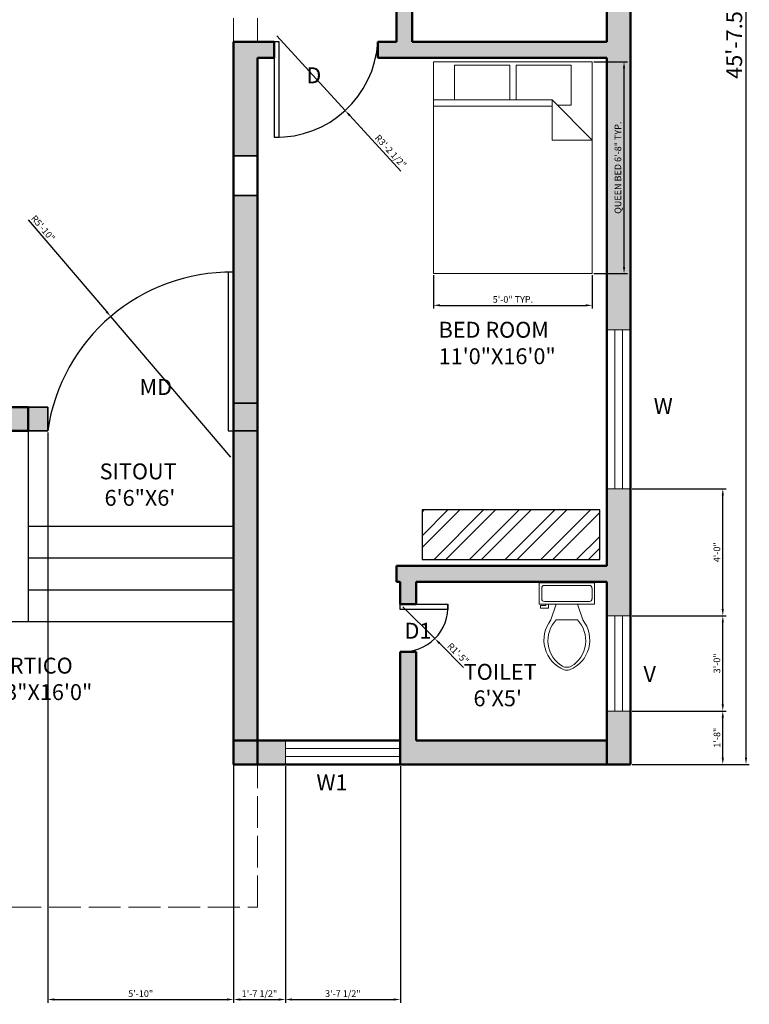
# Model space of a CAD drawing. Units: inches. Extents: x 5703 to 6226, y 10088 to 10813.
# Tile 2 of 5: x 5950 to 6226, y 10088 to 10460. Entities that reach past the tile are written whole.
import ezdxf

# ---------------------------------------------------------------- set-up
doc = ezdxf.new("R2010")
doc.units = ezdxf.units.IN
doc.linetypes.add('ACAD_ISO02W100', pattern=[15, 12, -3])
for name, color, linetype, lineweight in [('A-ANNO-DIMS', 2, 'Continuous', 18), ('A-ANNO-TEXT', 7, 'Continuous', 18), ('A-AREA-IDEN', 7, 'Continuous', 18), ('A-COLS', 7, 'Continuous', 35), ('A-COLS-PATT', 7, 'Continuous', 13), ('A-DOOR', 140, 'Continuous', 25), ('A-FLOR-CASE', 8, 'Continuous', 25), ('A-FLOR-CASE-PATT', 9, 'Continuous', 13), ('A-FLOR-FIXT', 8, 'Continuous', 18), ('A-FLOR-STRS', 7, 'Continuous', 25), ('A-FURN', 8, 'Continuous', 18), ('A-WALL', 7, 'Continuous', 50), ('A-WALL-PATT', 9, 'Continuous', 13)]:
    doc.layers.add(name, color=color, linetype=linetype, lineweight=lineweight)
for name, color, linetype, lineweight, true_color in [('A-GLAZ', 112, 'Continuous', 18, 0x1ce368), ('A-ROOF-OVHD', 30, 'ACAD_ISO02W100', 18, 0xf8991e), ('A-WALL-OVHD', 30, 'ACAD_ISO02W100', 18, 0xf8991e)]:
    doc.layers.add(name, color=color, linetype=linetype, lineweight=lineweight, true_color=true_color)
doc.styles.get("Standard").update_dxf_attribs({"font": 'arial.ttf'})
doc.dimstyles.new('ISO-25', dxfattribs={"dimtxt": 2.5, "dimasz": 2.5, "dimexe": 1.25, "dimexo": 0.625, "dimtad": 1, "dimlunit": 3, "dimtxsty": 'Standard', "dimcen": 2.5, "dimadec": 0, "dimazin": 0, "dimtfac": 1, "dimtmove": 0, "dimatfit": 3, "dimfxl": 1, "dimarcsym": 0})

# ---------------------------------------------------------------- blocks, each defined once
blk = doc.blocks.new('*D11')
at = {"layer": 'A-ANNO-DIMS', "color": 0, "lineweight": -2, "transparency": 16777216}
for p, q in [((6181.8, 10725.87), (6226.04, 10725.87)), ((6224.79, 10723.37), (6224.79, 10180.87)), ((6181.8, 10178.37), (6226.04, 10178.37))]:
    blk.add_line(p, q, dxfattribs=at)
at = {"layer": 'A-ANNO-DIMS', "color": 0, "transparency": 16777216}
for points in [[(6224.38, 10723.37), (6225.21, 10723.37), (6224.79, 10725.87)], [(6224.38, 10180.87), (6225.21, 10180.87), (6224.79, 10178.37)]]:
    blk.add_solid(points, dxfattribs=at)
at = {"layer": 'Defpoints', "color": 0, "transparency": 16777216}
for p in [(6181.18, 10725.87), (6181.18, 10178.37), (6224.79, 10178.37)]:
    blk.add_point(p, dxfattribs=at)
at = {"layer": 'A-ANNO-DIMS', "color": 0, "transparency": 16777216, "insert": (6221.12, 10452.12), "char_height": 6, "width": 12.5074, "attachment_point": 5, "rotation": 90}
blk.add_mtext('45\'-7.5"', dxfattribs=at)
blk = doc.blocks.new('Bed - Queen')
for p, q in [((0, -80.00003), (0, 0)), ((0, 0), (59.99999, 0)), ((59.99999, 0), (59.99999, -80.00003)), ((7.99999, -1.2), (28.79998, -1.2)), ((7.99999, -14.4), (7.99999, -1.2)), ((28.79998, -1.2), (28.79998, -14.4)), ((31.19999, -1.2), (51.99999, -1.2)), ((31.19999, -14.4), (31.19999, -1.2)), ((51.99999, -1.2), (51.99999, -16.4)), ((0, -14.4), (44.8, -14.4)), ((59.99999, -29.6), (44.8, -14.4)), ((44.8, -14.4), (44.8, -29.6)), ((44.8, -16.8), (0, -16.8)), ((51.99999, -16.4), (46.79936, -16.4)), ((44.8, -29.6), (59.99999, -29.6)), ((59.99999, -80.00003), (0, -80.00003))]:
    blk.add_line(p, q)
blk = doc.blocks.new('Toilet - top')
for p, q in [((9.5, -6), (9.5, -2)), ((-10, -8.5), (-8, -8.5)), ((-10, -9.5), (-10, -8.5)), ((-7, -9.5), (-10, -9.5)), ((-8, -8.5), (-8, -8)), ((-7, -8), (-7, -9.5)), ((-4, -8), (-6, -14)), ((4, -8), (6, -14)), ((4, -14), (-4, -14))]:
    blk.add_line(p, q)
blk.add_lwpolyline([(10.5, -8), (10.5, 0), (-10.5, 0), (-10.5, -8)], close=True)
for points in [[(-9.5, -2), (-9.5, -6)], [(8.5, -1), (-8.5, -1)], [(-8.5, -7), (8.5, -7)]]:
    blk.add_lwpolyline(points)
for centre, radius, start, end in [((-8.62, -1.88), 0.884, 81.8699, 188.1301), ((8.62, -1.88), 0.884, 351.8699, 98.1301), ((-8.62, -6.12), 0.884, 171.8699, 278.1301), ((8.62, -6.12), 0.884, 261.8699, 8.1301), ((3.52, -21.58), 12.17, 141.4691, 247.9714), ((4.2, -21.82), 11.33, 136.3677, 238.9468), ((-3.52, -21.58), 12.17, 292.0284, 38.5307), ((-4.2, -21.82), 11.33, 301.053, 43.6321), ((0, -27.88), 4, 245.7318, 294.2682), ((0, -29), 4, 254.8605, 285.1395)]:
    blk.add_arc(centre, radius, start, end)
blk = doc.blocks.new('WIN-60x9')
for p, q in [((9, 60), (0, 60)), ((0, 60), (0, 0)), ((3, 60), (3, 0)), ((6, 0), (6, 60)), ((9, 0), (9, 60)), ((0, 0), (9, 0))]:
    blk.add_line(p, q)
blk = doc.blocks.new('*D18')
at = {"layer": 'A-ANNO-DIMS', "color": 0, "lineweight": -2, "transparency": 16777216}
for p, q in [((6167.33, 10443.83), (6179.96, 10443.83)), ((6178.71, 10366.33), (6178.71, 10441.33)), ((6167.33, 10363.83), (6179.96, 10363.83))]:
    blk.add_line(p, q, dxfattribs=at)
at = {"layer": 'A-ANNO-DIMS', "color": 0, "transparency": 16777216}
for points in [[(6178.29, 10441.33), (6179.13, 10441.33), (6178.71, 10443.83)], [(6178.29, 10366.33), (6179.13, 10366.33), (6178.71, 10363.83)]]:
    blk.add_solid(points, dxfattribs=at)
at = {"layer": 'Defpoints', "color": 0, "transparency": 16777216}
for p in [(6166.71, 10443.83), (6178.71, 10443.83), (6166.71, 10363.83)]:
    blk.add_point(p, dxfattribs=at)
at = {"layer": 'A-ANNO-DIMS', "color": 0, "transparency": 16777216, "insert": (6176.71, 10403.83), "char_height": 2.5, "attachment_point": 5, "rotation": 90}
blk.add_mtext('QUEEN BED 6\'-8" TYP.', dxfattribs=at)
blk = doc.blocks.new('*D19')
at = {"layer": 'A-ANNO-DIMS', "color": 0, "lineweight": -2, "transparency": 16777216}
for p, q in [((6106.71, 10363.21), (6106.71, 10350.58)), ((6166.71, 10363.21), (6166.71, 10350.58)), ((6109.21, 10351.83), (6164.21, 10351.83))]:
    blk.add_line(p, q, dxfattribs=at)
at = {"layer": 'A-ANNO-DIMS', "color": 0, "transparency": 16777216}
for points in [[(6109.21, 10352.25), (6109.21, 10351.42), (6106.71, 10351.83)], [(6164.21, 10352.25), (6164.21, 10351.42), (6166.71, 10351.83)]]:
    blk.add_solid(points, dxfattribs=at)
at = {"layer": 'Defpoints', "color": 0, "transparency": 16777216}
for p in [(6106.71, 10363.83), (6166.71, 10363.83), (6166.71, 10351.83)]:
    blk.add_point(p, dxfattribs=at)
at = {"layer": 'A-ANNO-DIMS', "color": 0, "transparency": 16777216, "insert": (6136.71, 10353.73), "char_height": 2.5, "attachment_point": 5}
blk.add_mtext('5\'-0" TYP.', dxfattribs=at)
blk = doc.blocks.new('*D42')
at = {"layer": 'A-ANNO-DIMS', "color": 0, "lineweight": -2, "transparency": 16777216}
for p, q in [((5960.95, 10303.74), (5960.95, 10088.29)), ((6031.18, 10303.74), (6031.18, 10088.29)), ((5963.45, 10089.54), (6028.68, 10089.54))]:
    blk.add_line(p, q, dxfattribs=at)
at = {"layer": 'A-ANNO-DIMS', "color": 0, "transparency": 16777216}
for points in [[(5963.45, 10089.96), (5963.45, 10089.12), (5960.95, 10089.54)], [(6028.68, 10089.96), (6028.68, 10089.12), (6031.18, 10089.54)]]:
    blk.add_solid(points, dxfattribs=at)
at = {"layer": 'Defpoints', "color": 0, "transparency": 16777216}
for p in [(5960.95, 10304.37), (6031.18, 10304.37), (6031.18, 10089.54)]:
    blk.add_point(p, dxfattribs=at)
at = {"layer": 'A-ANNO-DIMS', "color": 0, "transparency": 16777216, "insert": (5996.07, 10091.44), "char_height": 2.5, "attachment_point": 5}
blk.add_mtext('5\'-10"', dxfattribs=at)
blk = doc.blocks.new('*D51')
at = {"layer": 'A-ANNO-DIMS', "color": 0, "lineweight": -2, "transparency": 16777216}
for p, q in [((6181.8, 10198.55), (6217.28, 10198.55)), ((6216.03, 10180.87), (6216.03, 10196.05)), ((6181.8, 10178.37), (6217.28, 10178.37))]:
    blk.add_line(p, q, dxfattribs=at)
at = {"layer": 'A-ANNO-DIMS', "color": 0, "transparency": 16777216}
for points in [[(6215.61, 10196.05), (6216.44, 10196.05), (6216.03, 10198.55)], [(6215.61, 10180.87), (6216.44, 10180.87), (6216.03, 10178.37)]]:
    blk.add_solid(points, dxfattribs=at)
at = {"layer": 'Defpoints', "color": 0, "transparency": 16777216}
for p in [(6181.18, 10198.55), (6216.03, 10198.55), (6181.18, 10178.37)]:
    blk.add_point(p, dxfattribs=at)
at = {"layer": 'A-ANNO-DIMS', "color": 0, "transparency": 16777216, "insert": (6214.12, 10188.46), "char_height": 2.5, "attachment_point": 5, "rotation": 90}
blk.add_mtext('1\'-8"', dxfattribs=at)
blk = doc.blocks.new('*D52')
at = {"layer": 'A-ANNO-DIMS', "color": 0, "lineweight": -2, "transparency": 16777216}
for p, q in [((6181.8, 10234.55), (6217.28, 10234.55)), ((6216.03, 10201.05), (6216.03, 10232.05)), ((6181.8, 10198.55), (6217.28, 10198.55))]:
    blk.add_line(p, q, dxfattribs=at)
at = {"layer": 'A-ANNO-DIMS', "color": 0, "transparency": 16777216}
for points in [[(6215.61, 10232.05), (6216.44, 10232.05), (6216.03, 10234.55)], [(6215.61, 10201.05), (6216.44, 10201.05), (6216.03, 10198.55)]]:
    blk.add_solid(points, dxfattribs=at)
at = {"layer": 'Defpoints', "color": 0, "transparency": 16777216}
for p in [(6181.18, 10234.55), (6216.03, 10234.55), (6181.18, 10198.55)]:
    blk.add_point(p, dxfattribs=at)
at = {"layer": 'A-ANNO-DIMS', "color": 0, "transparency": 16777216, "insert": (6214.12, 10216.55), "char_height": 2.5, "attachment_point": 5, "rotation": 90}
blk.add_mtext('3\'-0"', dxfattribs=at)
blk = doc.blocks.new('*D53')
at = {"layer": 'A-ANNO-DIMS', "color": 0, "lineweight": -2, "transparency": 16777216}
for p, q in [((6181.8, 10282.53), (6217.28, 10282.53)), ((6216.03, 10237.05), (6216.03, 10280.03)), ((6181.8, 10234.55), (6217.28, 10234.55))]:
    blk.add_line(p, q, dxfattribs=at)
at = {"layer": 'A-ANNO-DIMS', "color": 0, "transparency": 16777216}
for points in [[(6215.61, 10280.03), (6216.44, 10280.03), (6216.03, 10282.53)], [(6215.61, 10237.05), (6216.44, 10237.05), (6216.03, 10234.55)]]:
    blk.add_solid(points, dxfattribs=at)
at = {"layer": 'Defpoints', "color": 0, "transparency": 16777216}
for p in [(6181.18, 10282.53), (6216.03, 10282.53), (6181.18, 10234.55)]:
    blk.add_point(p, dxfattribs=at)
at = {"layer": 'A-ANNO-DIMS', "color": 0, "transparency": 16777216, "insert": (6214.12, 10258.54), "char_height": 2.5, "attachment_point": 5, "rotation": 90}
blk.add_mtext('4\'-0"', dxfattribs=at)
blk = doc.blocks.new('*D55')
at = {"layer": 'A-ANNO-DIMS', "color": 0, "lineweight": -2, "transparency": 16777216}
for p, q in [((6031.18, 10177.74), (6031.18, 10088.29)), ((6050.75, 10177.74), (6050.75, 10088.29)), ((6033.68, 10089.54), (6048.25, 10089.54))]:
    blk.add_line(p, q, dxfattribs=at)
at = {"layer": 'A-ANNO-DIMS', "color": 0, "transparency": 16777216}
for points in [[(6033.68, 10089.96), (6033.68, 10089.12), (6031.18, 10089.54)], [(6048.25, 10089.96), (6048.25, 10089.12), (6050.75, 10089.54)]]:
    blk.add_solid(points, dxfattribs=at)
at = {"layer": 'Defpoints', "color": 0, "transparency": 16777216}
for p in [(6031.18, 10178.37), (6050.75, 10178.37), (6050.75, 10089.54)]:
    blk.add_point(p, dxfattribs=at)
at = {"layer": 'A-ANNO-DIMS', "color": 0, "transparency": 16777216, "insert": (6040.96, 10091.46), "char_height": 2.5, "attachment_point": 5}
blk.add_mtext('1\'-7 1/2"', dxfattribs=at)
blk = doc.blocks.new('*D56')
at = {"layer": 'A-ANNO-DIMS', "color": 0, "lineweight": -2, "transparency": 16777216}
for p, q in [((6050.75, 10177.74), (6050.75, 10088.29)), ((6094.18, 10177.74), (6094.18, 10088.29)), ((6053.25, 10089.54), (6091.68, 10089.54))]:
    blk.add_line(p, q, dxfattribs=at)
at = {"layer": 'A-ANNO-DIMS', "color": 0, "transparency": 16777216}
for points in [[(6053.25, 10089.96), (6053.25, 10089.12), (6050.75, 10089.54)], [(6091.68, 10089.96), (6091.68, 10089.12), (6094.18, 10089.54)]]:
    blk.add_solid(points, dxfattribs=at)
at = {"layer": 'Defpoints', "color": 0, "transparency": 16777216}
for p in [(6050.75, 10178.37), (6094.18, 10178.37), (6094.18, 10089.54)]:
    blk.add_point(p, dxfattribs=at)
at = {"layer": 'A-ANNO-DIMS', "color": 0, "transparency": 16777216, "insert": (6072.46, 10091.46), "char_height": 2.5, "attachment_point": 5}
blk.add_mtext('3\'-7 1/2"', dxfattribs=at)
blk = doc.blocks.new('*D60')
at = {"layer": 'A-ANNO-DIMS', "color": 0, "lineweight": -2, "transparency": 16777216}
for p, q in [((6047.46, 10453.63), (6073.34, 10425.44)), ((6094.33, 10402.58), (6075.04, 10423.6))]:
    blk.add_line(p, q, dxfattribs=at)
at = {"layer": 'A-ANNO-DIMS', "color": 0, "transparency": 16777216}
blk.add_solid([(6075.34, 10423.88), (6074.73, 10423.31), (6073.34, 10425.44)], dxfattribs=at)
at = {"layer": 'Defpoints', "color": 0, "transparency": 16777216}
for p in [(6047.46, 10453.63), (6073.34, 10425.44)]:
    blk.add_point(p, dxfattribs=at)
at = {"layer": 'A-ANNO-DIMS', "color": 0, "transparency": 16777216, "insert": (6090.29, 10409.82), "char_height": 2.5, "attachment_point": 5, "rotation": 312.5558}
blk.add_mtext('R3\'-2 1/2"', dxfattribs=at)
blk = doc.blocks.new('*D61')
at = {"layer": 'A-ANNO-DIMS', "color": 0, "lineweight": -2, "transparency": 16777216}
for p, q in [((6095.18, 10237.95), (6107.22, 10225.91)), ((6118.08, 10215.05), (6108.99, 10224.15))]:
    blk.add_line(p, q, dxfattribs=at)
at = {"layer": 'A-ANNO-DIMS', "color": 0, "transparency": 16777216}
blk.add_solid([(6109.28, 10224.44), (6108.69, 10223.85), (6107.22, 10225.91)], dxfattribs=at)
at = {"layer": 'Defpoints', "color": 0, "transparency": 16777216}
for p in [(6095.18, 10237.95), (6107.22, 10225.91)]:
    blk.add_point(p, dxfattribs=at)
at = {"layer": 'A-ANNO-DIMS', "color": 0, "transparency": 16777216, "insert": (6115.79, 10220.03), "char_height": 2.5, "attachment_point": 5, "rotation": 315.0011}
blk.add_mtext('R1\'-5"', dxfattribs=at)
blk = doc.blocks.new('*D62')
at = {"layer": 'A-ANNO-DIMS', "color": 0, "lineweight": -2, "transparency": 16777216}
for p, q in [((5953.52, 10384.16), (5983.13, 10349.51)), ((6030.18, 10294.45), (5984.75, 10347.61))]:
    blk.add_line(p, q, dxfattribs=at)
at = {"layer": 'A-ANNO-DIMS', "color": 0, "transparency": 16777216}
blk.add_solid([(5983.44, 10349.78), (5982.81, 10349.24), (5984.75, 10347.61)], dxfattribs=at)
at = {"layer": 'Defpoints', "color": 0, "transparency": 16777216}
for p in [(5984.75, 10347.61), (6030.18, 10294.45)]:
    blk.add_point(p, dxfattribs=at)
at = {"layer": 'A-ANNO-DIMS', "color": 0, "transparency": 16777216, "insert": (5958.94, 10380.75), "char_height": 2.5, "attachment_point": 5, "rotation": 310.5118}
blk.add_mtext('R5\'-10"', dxfattribs=at)

msp = doc.modelspace()

# ---------------------------------------------------------------- hatches: boundary and pattern name
at = {"layer": 'A-COLS-PATT'}
h = msp.add_hatch(color=256, dxfattribs=at)
h.dxf.hatch_style = 1
h.paths.add_polyline_path([(5788.176, 10725.869), (5773.176, 10725.869), (5773.176, 10716.869), (5788.176, 10716.869)])
h.paths.add_polyline_path([(5782.176, 10516.684), (5773.176, 10516.684), (5773.176, 10497.849), (5782.176, 10497.849)])
h.paths.add_polyline_path([(5782.176, 10319.369), (5773.176, 10319.369), (5773.176, 10304.369), (5782.176, 10304.369)])
h.paths.add_polyline_path([(5960.955, 10313.369), (5953.525, 10313.369), (5953.525, 10304.369), (5960.955, 10304.369)])
h.paths.add_polyline_path([(6040.176, 10314.869), (6031.176, 10314.869), (6031.176, 10304.369), (6040.176, 10304.369)])
h.paths.add_polyline_path([(6181.176, 10198.545), (6172.176, 10198.545), (6172.176, 10178.369), (6181.176, 10178.369)])
h.paths.add_polyline_path([(6181.176, 10505.369), (6172.176, 10505.369), (6172.176, 10492.633), (6181.176, 10492.633)])
h.paths.add_polyline_path([(6181.176, 10725.869), (6166.176, 10725.869), (6166.176, 10716.869), (6181.176, 10716.869)])
at = {"layer": 'A-FLOR-CASE-PATT'}
h = msp.add_hatch(dxfattribs=at)
h.set_pattern_fill('ANSI32', color=256)
h.paths.add_polyline_path([(6169.528, 10274.524), (6102.412, 10274.524), (6102.412, 10255.78), (6169.528, 10255.78)])
at = {"layer": 'A-WALL-PATT'}
h = msp.add_hatch(color=256, dxfattribs=at)
h.dxf.hatch_style = 1
h.paths.add_polyline_path([(6057.982, 10725.869), (6040.176, 10725.869), (6040.176, 10749.869), (5999.271, 10749.869), (5999.271, 10740.869), (6031.176, 10740.869), (6031.176, 10716.869), (6031.176, 10511.369), (6013.525, 10511.369), (6013.525, 10505.369), (6048.161, 10505.369), (6048.161, 10511.369), (6040.176, 10511.369), (6040.176, 10716.869), (6057.982, 10716.869)])
h.paths.add_polyline_path([(6166.176, 10725.869), (6093.982, 10725.869), (6093.982, 10716.869), (6166.176, 10716.869)])
h.paths.add_polyline_path([(6181.176, 10716.869), (6172.176, 10716.869), (6172.176, 10511.369), (6132.161, 10511.369, -0.0172363), (6132.161, 10509.369), (6132.161, 10505.369), (6181.176, 10505.369)])
h.paths.add_polyline_path([(6181.176, 10468.633), (6172.176, 10468.633), (6172.176, 10451.369), (6098.676, 10451.369), (6098.676, 10505.369), (6102.161, 10505.369), (6102.161, 10511.369), (6090.161, 10511.369), (6090.161, 10507.369, -0.0121933), (6090.161, 10505.369), (6092.676, 10505.369), (6092.676, 10451.369), (6085.668, 10451.369), (6085.668, 10445.369), (6092.676, 10445.369), (6172.176, 10445.369), (6172.176, 10342.529), (6181.176, 10342.529)])
h.paths.add_polyline_path([(6181.176, 10282.529), (6172.176, 10282.529), (6172.176, 10253.369), (6092.676, 10253.369), (6092.676, 10247.369), (6094.176, 10247.369), (6094.176, 10238.954), (6100.176, 10238.954), (6100.176, 10247.369), (6172.176, 10247.369), (6172.176, 10234.545), (6181.176, 10234.545)])
h.paths.add_polyline_path([(6172.176, 10187.369), (6100.176, 10187.369), (6100.176, 10220.954), (6096.176, 10220.954, -0.0293864), (6094.176, 10220.954), (6094.176, 10178.369), (6172.176, 10178.369)])
h.paths.add_polyline_path([(6050.745, 10187.369), (6040.176, 10187.369), (6040.176, 10178.369), (6050.745, 10178.369)])
h.paths.add_polyline_path([(6040.176, 10187.369), (6031.176, 10187.369), (6031.176, 10178.369), (6040.176, 10178.369)])
h.paths.add_polyline_path([(6040.176, 10304.369), (6031.176, 10304.369), (6031.176, 10187.369), (6040.176, 10187.369)])
h.paths.add_polyline_path([(6040.176, 10393.328), (6031.176, 10393.328), (6031.176, 10314.869), (6040.176, 10314.869)])
h.paths.add_polyline_path([(6040.176, 10445.369), (6046.458, 10445.369), (6046.458, 10451.369), (6031.176, 10451.369), (6031.176, 10408.328), (6040.176, 10408.328)])
h.paths.add_polyline_path([(5911.176, 10584.869), (5845.666, 10584.869, -0.0172363), (5845.666, 10582.869), (5845.666, 10578.869), (5902.176, 10578.869), (5902.176, 10505.369), (5953.525, 10505.369), (5953.525, 10511.369), (5911.176, 10511.369)])
h.paths.add_polyline_path([(5902.176, 10511.369), (5782.176, 10511.369), (5782.176, 10505.369), (5902.176, 10505.369)])
h.paths.add_polyline_path([(5782.176, 10578.869), (5815.666, 10578.869), (5815.666, 10584.869), (5773.176, 10584.869), (5773.176, 10516.684), (5782.176, 10516.684)])
h.paths.add_polyline_path([(5782.176, 10497.849), (5773.176, 10497.849), (5773.176, 10438.429), (5782.176, 10438.429)])
h.paths.add_polyline_path([(5782.176, 10378.429), (5773.176, 10378.429), (5773.176, 10319.369), (5782.176, 10319.369)])
h.paths.add_polyline_path([(5824.846, 10313.369), (5782.176, 10313.369), (5782.176, 10304.369), (5824.846, 10304.369)])
h.paths.add_polyline_path([(5953.525, 10313.369), (5872.846, 10313.369), (5872.846, 10304.369), (5953.525, 10304.369)])

# ---------------------------------------------------------------- linework, layer by layer
at = {"layer": 'A-COLS'}
for p, q in [((6031.176, 10408.328), (6040.176, 10408.328)), ((6031.176, 10408.328), (6031.176, 10402.328)), ((6040.176, 10393.328), (6040.176, 10408.328)), ((6031.176, 10402.328), (6031.176, 10393.328)), ((6031.176, 10393.328), (6040.176, 10393.328)), ((5953.525, 10313.369), (5953.525, 10304.369)), ((5960.955, 10313.369), (5953.525, 10313.369)), ((5960.955, 10313.369), (5960.955, 10304.369)), ((6031.176, 10304.369), (6031.176, 10314.869)), ((6031.176, 10314.869), (6040.176, 10314.869)), ((6040.176, 10314.869), (6040.176, 10304.369)), ((5953.525, 10304.369), (5960.955, 10304.369)), ((6031.176, 10304.369), (6040.176, 10304.369))]:
    msp.add_line(p, q, dxfattribs=at)
at = {"layer": 'A-DOOR'}
for p, q in [((6046.458, 10451.369), (6046.458, 10415.369)), ((6048.458, 10451.369), (6046.458, 10451.369)), ((6048.458, 10415.369), (6048.458, 10451.369)), ((6046.458, 10415.369), (6048.458, 10415.369)), ((6031.176, 10364.369), (6029.176, 10364.369)), ((6029.176, 10364.369), (6029.176, 10304.369)), ((6031.176, 10304.369), (6031.176, 10364.369)), ((6029.176, 10304.369), (6031.176, 10304.369)), ((6094.176, 10238.954), (6112.176, 10238.954)), ((6094.176, 10236.954), (6094.176, 10238.954)), ((6112.176, 10238.954), (6112.176, 10236.954)), ((6112.176, 10236.954), (6094.176, 10236.954))]:
    msp.add_line(p, q, dxfattribs=at)
for centre, radius, start, end in [((6047.458, 10453.633), 38.277, 268.50295, 356.60932), ((6030.176, 10294.447), 69.929, 89.18063, 171.84304), ((6095.176, 10237.954), 17.029, 266.63354, 3.36646)]:
    msp.add_arc(centre, radius, start, end, dxfattribs=at)
at = {"layer": 'A-FLOR-CASE'}
msp.add_lwpolyline([(6102.412, 10255.78), (6169.528, 10255.78), (6169.528, 10274.524), (6102.412, 10274.524)], close=True, dxfattribs=at)
at = {"layer": 'A-FLOR-STRS'}
for p, q in [((5953.525, 10304.369), (5953.525, 10232.369)), ((5953.525, 10268.369), (6031.176, 10268.369)), ((5953.525, 10256.369), (6031.176, 10256.369)), ((5953.525, 10244.369), (6031.176, 10244.369)), ((5947.176, 10232.369), (5953.525, 10232.369)), ((5953.525, 10232.369), (6031.176, 10232.369))]:
    msp.add_line(p, q, dxfattribs=at)
at = {"layer": 'A-GLAZ'}
for p, q in [((6172.176, 10234.545), (6181.176, 10234.545)), ((6172.176, 10234.545), (6172.176, 10210.545)), ((6175.176, 10234.545), (6175.176, 10210.545)), ((6178.176, 10234.545), (6178.176, 10210.545)), ((6181.176, 10198.545), (6181.176, 10234.545)), ((6172.176, 10210.545), (6172.176, 10198.545)), ((6175.176, 10210.545), (6175.176, 10198.545)), ((6178.176, 10210.545), (6178.176, 10198.545)), ((6172.176, 10198.545), (6181.176, 10198.545)), ((6050.745, 10187.369), (6050.745, 10178.369)), ((6050.745, 10187.369), (6094.176, 10187.369)), ((6094.176, 10187.369), (6094.176, 10178.369)), ((6050.745, 10184.369), (6094.176, 10184.369)), ((6050.745, 10181.369), (6094.176, 10181.369)), ((6050.745, 10178.369), (6094.176, 10178.369))]:
    msp.add_line(p, q, dxfattribs=at)
at = {"layer": 'A-ROOF-OVHD'}
for p, q in [((6040.176, 10124.389), (6040.176, 10178.369)), ((5751.498, 10124.389), (6040.176, 10124.389))]:
    msp.add_line(p, q, dxfattribs=at)
at = {"layer": 'A-WALL'}
for p, q in [((6092.676, 10451.369), (6092.676, 10505.369)), ((6098.676, 10451.369), (6098.676, 10505.369)), ((6172.176, 10451.369), (6172.176, 10468.633)), ((6181.176, 10178.369), (6181.176, 10468.633)), ((6031.176, 10178.369), (6031.176, 10451.369)), ((6031.176, 10451.369), (6046.458, 10451.369)), ((6046.458, 10451.369), (6046.458, 10445.369)), ((6085.668, 10445.369), (6085.668, 10451.369)), ((6085.668, 10451.369), (6092.676, 10451.369)), ((6098.676, 10451.369), (6172.176, 10451.369)), ((6040.176, 10178.369), (6040.176, 10445.369)), ((6040.176, 10445.369), (6046.458, 10445.369)), ((6092.676, 10445.369), (6085.668, 10445.369)), ((6092.676, 10445.369), (6172.176, 10445.369)), ((6172.176, 10253.369), (6172.176, 10445.369)), ((5782.176, 10313.369), (5953.525, 10313.369)), ((5953.525, 10313.369), (5953.525, 10304.369)), ((5773.176, 10304.369), (5953.525, 10304.369)), ((6092.676, 10253.369), (6172.176, 10253.369)), ((6092.676, 10253.369), (6092.676, 10247.369)), ((6092.676, 10247.369), (6094.176, 10247.369)), ((6094.176, 10238.954), (6094.176, 10247.369)), ((6100.176, 10247.369), (6172.176, 10247.369)), ((6100.176, 10238.954), (6100.176, 10247.369)), ((6172.176, 10178.369), (6172.176, 10247.369)), ((6094.176, 10238.954), (6100.176, 10238.954)), ((6094.176, 10178.369), (6094.176, 10220.954)), ((6094.176, 10220.954), (6100.176, 10220.954)), ((6100.176, 10187.369), (6100.176, 10220.954)), ((6094.176, 10187.369), (6031.176, 10187.369)), ((6100.176, 10187.369), (6172.176, 10187.369)), ((6094.176, 10178.369), (6031.176, 10178.369)), ((6094.176, 10178.369), (6181.176, 10178.369))]:
    msp.add_line(p, q, dxfattribs=at)
at = {"layer": 'A-WALL-OVHD'}
for p, q in [((6031.176, 10505.369), (6031.176, 10451.369)), ((6040.176, 10505.369), (6040.176, 10451.369))]:
    msp.add_line(p, q, dxfattribs=at)

# ---------------------------------------------------------------- block references
at = {"layer": 'A-FLOR-FIXT'}
msp.add_blockref('Toilet - top', (6157.105, 10246.956), dxfattribs=at)
at = {"layer": 'A-FURN'}
msp.add_blockref('Bed - Queen', (6106.709, 10443.832), dxfattribs=at)
at = {"layer": 'A-GLAZ'}
msp.add_blockref('WIN-60x9', (6172.176, 10282.529), dxfattribs=at)

# ---------------------------------------------------------------- texts
at = {"layer": 'A-ANNO-TEXT', "char_height": 6, "attachment_point": 1}
for s, insert in [(' D', (6056.834, 10441.733)), (' MD', (5993.795, 10323.965)), (' W', (6188.092, 10316.803)), (' D1', (6093.935, 10231.872)), (' V', (6184.219, 10215.533)), ('W1', (6062.482, 10174.574))]:
    msp.add_mtext_dynamic_manual_height_columns(s, width=71.13425, gutter_width=12.5, heights=[0], dxfattribs=dict(at, insert=insert))
at = {"layer": 'A-AREA-IDEN', "char_height": 6, "attachment_point": 1}
for s, insert in [(' BED ROOM\\P 11\'0"X16\'0"', (6106.81, 10345.601)), ('SITOUT\\P 6\'6"X6\'', (5980.57, 10292.087)), (' PORTICO\\P16\'3"X16\'0"', (5933.505, 10218.693)), (" TOILET\\P   6'X5'", (6116.312, 10216.346))]:
    msp.add_mtext_dynamic_manual_height_columns(s, width=71.13425, gutter_width=12.5, heights=[0], dxfattribs=dict(at, insert=insert))

# ---------------------------------------------------------------- dimensions: what is measured, and where the dimension line sits
at = {"layer": 'A-ANNO-DIMS'}
for base, p1, p2, override, picture, middle in [((6224.795, 10178.369), (6181.176, 10725.869), (6181.176, 10178.369), {"dimtxt": 6, "dimclrd": 0, "dimclre": 0, "dimclrt": 0}, '*D11', (6221.118, 10452.119)), ((6216.026, 10282.529), (6181.176, 10234.545), (6181.176, 10282.529), {"dimdec": 1, "dimlfac": 1, "dimrnd": 0, "dimzin": 1, "dimdsep": 46, "dimlunit": 4, "dimfrac": 2}, '*D53', (6214.125, 10258.537)), ((6216.026, 10234.545), (6181.176, 10198.545), (6181.176, 10234.545), {"dimdec": 1, "dimlfac": 1, "dimrnd": 0, "dimzin": 1, "dimdsep": 46, "dimlunit": 4, "dimfrac": 2}, '*D52', (6214.124, 10216.545)), ((6216.026, 10198.545), (6181.176, 10178.369), (6181.176, 10198.545), {"dimdec": 1, "dimlfac": 1, "dimrnd": 0, "dimzin": 1, "dimdsep": 46, "dimlunit": 4, "dimfrac": 2}, '*D51', (6214.125, 10188.457))]:
    dim = msp.add_linear_dim(base=base, p1=p1, p2=p2, angle=90, dimstyle='ISO-25', override=override, dxfattribs=at)
    dim.commit()
    dim.dimension.update_dxf_attribs({"geometry": picture, "text_midpoint": middle})
for center, mpoint, picture, middle in [((6047.458, 10453.633), (6073.345, 10425.437), '*D60', (6088.877, 10408.52)), ((6030.176, 10294.447), (5984.75, 10347.612), '*D62', (5957.494, 10379.511)), ((6095.176, 10237.954), (6107.218, 10225.913), '*D61', (6114.443, 10218.688))]:
    dim = msp.add_radius_dim(center=center, mpoint=mpoint, dimstyle='ISO-25', override={"dimdec": 1, "dimlfac": 1, "dimrnd": 0, "dimzin": 1, "dimdsep": 46, "dimlunit": 4, "dimfrac": 2}, dxfattribs=at)
    dim.commit()
    dim.dimension.update_dxf_attribs({"geometry": picture, "text_midpoint": middle, "dimtype": 164})
dim = msp.add_linear_dim(base=(6178.709, 10443.832), p1=(6166.709, 10363.832), p2=(6166.709, 10443.832), angle=90, text='QUEEN BED <> TYP.', dimstyle='ISO-25', override={"dimdec": 1, "dimlfac": 1, "dimrnd": 0, "dimzin": 1, "dimdsep": 46, "dimlunit": 4, "dimfrac": 2}, dxfattribs=at)
dim.commit()
dim.dimension.update_dxf_attribs({"geometry": '*D18', "text_midpoint": (6176.715, 10403.832)})
dim = msp.add_linear_dim(base=(6166.709, 10351.832), p1=(6106.709, 10363.832), p2=(6166.709, 10363.832), text='<> TYP.', dimstyle='ISO-25', override={"dimdec": 1, "dimlfac": 1, "dimrnd": 0, "dimzin": 1, "dimdsep": 46, "dimlunit": 4, "dimfrac": 2}, dxfattribs=at)
dim.commit()
dim.dimension.update_dxf_attribs({"geometry": '*D19', "text_midpoint": (6136.709, 10353.733)})
for base, p1, p2, picture, middle in [((6031.176, 10089.539), (5960.955, 10304.369), (6031.176, 10304.369), '*D42', (5996.066, 10091.441)), ((6050.745, 10089.539), (6031.176, 10178.369), (6050.745, 10178.369), '*D55', (6040.961, 10091.457)), ((6094.176, 10089.539), (6050.745, 10178.369), (6094.176, 10178.369), '*D56', (6072.461, 10091.458))]:
    dim = msp.add_linear_dim(base=base, p1=p1, p2=p2, dimstyle='ISO-25', override={"dimdec": 1, "dimlfac": 1, "dimrnd": 0, "dimzin": 1, "dimdsep": 46, "dimlunit": 4, "dimfrac": 2}, dxfattribs=at)
    dim.commit()
    dim.dimension.update_dxf_attribs({"geometry": picture, "text_midpoint": middle})

doc.saveas('drawing.dxf')
